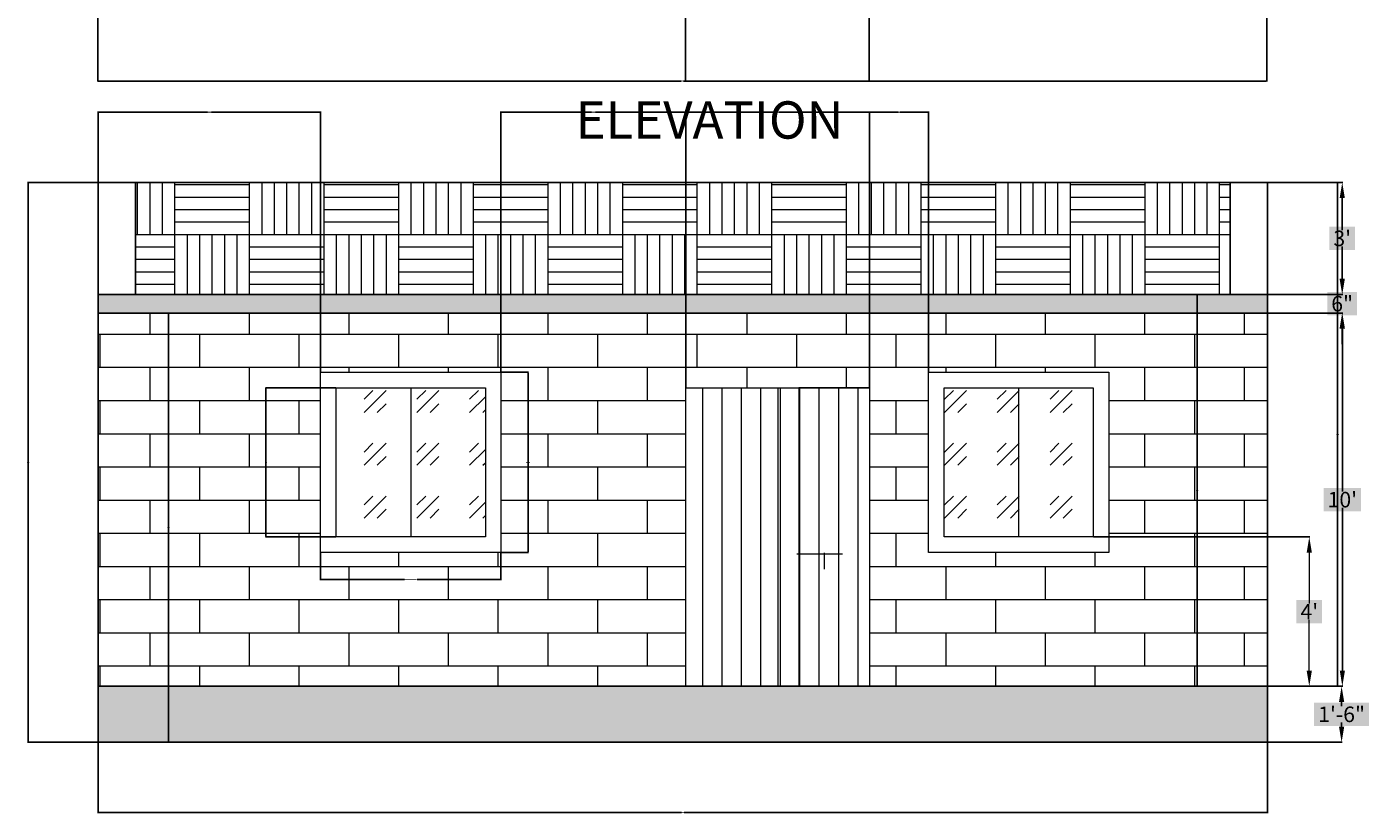
# Model space of a CAD drawing. Units: inches. Extents: x -35 to 832, y -515 to 219.
# Tile 1 of 7: x -33 to 399, y -515 to -262. Entities that reach past the tile are written whole.
import ezdxf

# ---------------------------------------------------------------- set-up
doc = ezdxf.new("R2010")
doc.units = ezdxf.units.IN
doc.header["$MEASUREMENT"] = 0
for name, color, linetype, lineweight in [('A-ANNO-DIMS', 2, 'Continuous', 18), ('A-ELEV', 3, 'Continuous', 25), ('A-ELEV-DOOR', 4, 'Continuous', 18), ('A-ELEV-GLAZ', 4, 'Continuous', 18), ('A-ELEV-PATT', 4, 'Continuous', 13), ('G-ANNO-TEXT', 7, 'Continuous', 35), ('S-ANNO-DIMS', 2, 'Continuous', 18)]:
    doc.layers.add(name, color=color, linetype=linetype, lineweight=lineweight)
doc.styles.get("Standard").update_dxf_attribs({"font": 'arial.ttf'})
doc.dimstyles.get("Standard").update_dxf_attribs({"dimtxt": 0.18, "dimasz": 0.18, "dimexe": 0.18, "dimexo": 0.0625, "dimgap": 0.09, "dimtad": 0, "dimtih": 1, "dimtoh": 1, "dimdec": 1, "dimzin": 0, "dimdsep": 46, "dimlunit": 4, "dimtxsty": 'Standard', "dimcen": 0.09, "dimclrd": 211, "dimclre": 4, "dimclrt": 3, "dimadec": 0, "dimazin": 0, "dimtfac": 0.5, "dimtdec": 1, "dimtofl": 0, "dimtmove": 0, "dimatfit": 3, "dimfxl": 1, "dimtfill": 2, "dimtfillclr": 61, "dimtolj": 1, "dimtzin": 0, "dimarcsym": 0})

# ---------------------------------------------------------------- blocks, each defined once
blk = doc.blocks.new('*D23')
at = {"layer": 'A-ANNO-DIMS', "color": 0, "lineweight": -2, "transparency": 16777216}
for p, q in [((366.05, -474.29), (390.03, -474.29)), ((389.85, -479.29), (389.85, -480.65)), ((389.85, -487.29), (389.85, -485.93)), ((366.05, -492.29), (390.03, -492.29))]:
    blk.add_line(p, q, dxfattribs=at)
at = {"layer": 'A-ANNO-DIMS', "color": 0, "transparency": 16777216}
for points in [[(389.02, -479.29), (390.68, -479.29), (389.85, -474.29)], [(389.02, -487.29), (390.68, -487.29), (389.85, -492.29)]]:
    blk.add_solid(points, dxfattribs=at)
at = {"layer": 'Defpoints', "color": 0, "transparency": 16777216}
for p in [(365.98, -474.29), (389.85, -474.29), (365.98, -492.29)]:
    blk.add_point(p, dxfattribs=at)
at = {"layer": 'A-ANNO-DIMS', "color": 0, "transparency": 16777216, "insert": (389.85, -483.29), "char_height": 5, "attachment_point": 5, "bg_fill": 1, "box_fill_scale": 1.25, "bg_fill_color": 61, "bg_fill_transparency": 0}
blk.add_mtext('\\A1;1\'-6"', dxfattribs=at)
blk = doc.blocks.new('*D24')
at = {"layer": 'A-ANNO-DIMS', "color": 0, "lineweight": -2, "transparency": 16777216}
for p, q in [((366.05, -354.29), (390.27, -354.29)), ((390.09, -359.29), (390.09, -411.65)), ((390.09, -469.29), (390.09, -416.93)), ((366.05, -474.29), (390.27, -474.29))]:
    blk.add_line(p, q, dxfattribs=at)
at = {"layer": 'A-ANNO-DIMS', "color": 0, "transparency": 16777216}
for points in [[(389.26, -359.29), (390.92, -359.29), (390.09, -354.29)], [(389.26, -469.29), (390.92, -469.29), (390.09, -474.29)]]:
    blk.add_solid(points, dxfattribs=at)
at = {"layer": 'Defpoints', "color": 0, "transparency": 16777216}
for p in [(365.98, -354.29), (390.09, -354.29), (365.98, -474.29)]:
    blk.add_point(p, dxfattribs=at)
at = {"layer": 'A-ANNO-DIMS', "color": 0, "transparency": 16777216, "insert": (390.09, -414.29), "char_height": 5, "attachment_point": 5, "bg_fill": 1, "box_fill_scale": 1.25, "bg_fill_color": 61, "bg_fill_transparency": 0}
blk.add_mtext("\\A1;10'", dxfattribs=at)
blk = doc.blocks.new('*D25')
at = {"layer": 'A-ANNO-DIMS', "color": 0, "lineweight": -2, "transparency": 16777216}
for p, q in [((390.03, -343.29), (390.03, -338.29)), ((366.05, -348.29), (390.21, -348.29)), ((366.05, -354.29), (390.21, -354.29)), ((390.03, -359.29), (390.03, -364.29))]:
    blk.add_line(p, q, dxfattribs=at)
at = {"layer": 'A-ANNO-DIMS', "color": 0, "transparency": 16777216}
for points in [[(389.2, -343.29), (390.87, -343.29), (390.03, -348.29)], [(389.2, -359.29), (390.87, -359.29), (390.03, -354.29)]]:
    blk.add_solid(points, dxfattribs=at)
at = {"layer": 'Defpoints', "color": 0, "transparency": 16777216}
for p in [(365.98, -348.29), (390.03, -348.29), (365.98, -354.29)]:
    blk.add_point(p, dxfattribs=at)
at = {"layer": 'A-ANNO-DIMS', "color": 0, "transparency": 16777216, "insert": (390.03, -351.29), "char_height": 5, "attachment_point": 5, "bg_fill": 1, "box_fill_scale": 1.25, "bg_fill_color": 61, "bg_fill_transparency": 0}
blk.add_mtext('\\A1;6"', dxfattribs=at)
blk = doc.blocks.new('*D26')
at = {"layer": 'A-ANNO-DIMS', "color": 0, "lineweight": -2, "transparency": 16777216}
for p, q in [((366.05, -312.29), (390.24, -312.29)), ((390.06, -317.29), (390.06, -327.64)), ((390.06, -343.29), (390.06, -332.93)), ((366.05, -348.29), (390.24, -348.29))]:
    blk.add_line(p, q, dxfattribs=at)
at = {"layer": 'A-ANNO-DIMS', "color": 0, "transparency": 16777216}
for points in [[(389.23, -317.29), (390.89, -317.29), (390.06, -312.29)], [(389.23, -343.29), (390.89, -343.29), (390.06, -348.29)]]:
    blk.add_solid(points, dxfattribs=at)
at = {"layer": 'Defpoints', "color": 0, "transparency": 16777216}
for p in [(365.98, -312.29), (390.06, -312.29), (365.98, -348.29)]:
    blk.add_point(p, dxfattribs=at)
at = {"layer": 'A-ANNO-DIMS', "color": 0, "transparency": 16777216, "insert": (390.06, -330.29), "char_height": 5, "attachment_point": 5, "bg_fill": 1, "box_fill_scale": 1.25, "bg_fill_color": 61, "bg_fill_transparency": 0}
blk.add_mtext("\\A1;3'", dxfattribs=at)
blk = doc.blocks.new('*D27')
at = {"layer": 'A-ANNO-DIMS', "color": 0, "lineweight": -2, "transparency": 16777216}
for p, q in [((310.05, -426.29), (379.64, -426.29)), ((311.18, -474.29), (379.64, -474.29))]:
    blk.add_line(p, q, dxfattribs=at)
at = {"layer": 'A-ANNO-DIMS', "color": 0, "lineweight": 13, "transparency": 16777216}
for p, q in [((379.46, -431.29), (379.46, -447.7)), ((379.46, -469.29), (379.46, -452.88))]:
    blk.add_line(p, q, dxfattribs=at)
at = {"layer": 'A-ANNO-DIMS', "color": 0, "transparency": 16777216}
for points in [[(378.62, -431.29), (380.29, -431.29), (379.46, -426.29)], [(378.62, -469.29), (380.29, -469.29), (379.46, -474.29)]]:
    blk.add_solid(points, dxfattribs=at)
at = {"layer": 'Defpoints', "color": 0, "transparency": 16777216}
for p in [(309.98, -426.29), (311.12, -474.29), (379.46, -474.29)]:
    blk.add_point(p, dxfattribs=at)
at = {"layer": 'A-ANNO-DIMS', "color": 0, "transparency": 16777216, "insert": (379.46, -450.29), "char_height": 5, "attachment_point": 5, "bg_fill": 1, "box_fill_scale": 1.25, "bg_fill_color": 61, "bg_fill_transparency": 0}
blk.add_mtext("\\A1;4'", dxfattribs=at)
blk = doc.blocks.new('WIN-48-ELEV')
blk.add_line((29, 53), (29, 5))
for points in [[(0, 58), (58, 58), (58, 0), (0, 0)], [(5, 53), (53, 53), (53, 5), (5, 5)]]:
    blk.add_lwpolyline(points, close=True)
blk = doc.blocks.new('*D69')
at = {"layer": 'Defpoints', "color": 0, "transparency": 16777216}
for p in [(61.48, -431.29), (119.48, -431.29), (119.48, -439.99)]:
    blk.add_point(p, dxfattribs=at)
at = {"layer": 'S-ANNO-DIMS', "color": 4, "lineweight": -2, "transparency": 16777216}
for p, q in [((61.48, -431.35), (61.48, -440.17)), ((119.48, -431.35), (119.48, -440.17))]:
    blk.add_line(p, q, dxfattribs=at)
at = {"layer": 'S-ANNO-DIMS', "color": 211, "lineweight": -2, "transparency": 16777216}
for p, q in [((61.66, -439.99), (88.42, -439.99)), ((119.3, -439.99), (92.54, -439.99))]:
    blk.add_line(p, q, dxfattribs=at)
at = {"layer": 'S-ANNO-DIMS', "color": 211, "transparency": 16777216}
for points in [[(61.66, -439.96), (61.66, -440.02), (61.48, -439.99)], [(119.3, -439.96), (119.3, -440.02), (119.48, -439.99)]]:
    blk.add_solid(points, dxfattribs=at)
at = {"layer": 'S-ANNO-DIMS', "color": 3, "transparency": 16777216, "insert": (90.48, -439.99), "char_height": 0.18, "attachment_point": 5, "bg_fill": 1, "box_fill_scale": 1.25, "bg_fill_color": 61, "bg_fill_transparency": 0}
blk.add_mtext('\\A1;WINDOW SURROUND 4\'-10" TYP.', dxfattribs=at)
blk = doc.blocks.new('*D70')
at = {"layer": 'Defpoints', "color": 0, "transparency": 16777216}
for p in [(119.48, -373.29), (128.18, -373.29), (119.48, -431.29)]:
    blk.add_point(p, dxfattribs=at)
at = {"layer": 'S-ANNO-DIMS', "color": 4, "lineweight": -2, "transparency": 16777216}
for p, q in [((119.55, -373.29), (128.36, -373.29)), ((119.55, -431.29), (128.36, -431.29))]:
    blk.add_line(p, q, dxfattribs=at)
at = {"layer": 'S-ANNO-DIMS', "color": 211, "lineweight": -2, "transparency": 16777216}
for p, q in [((128.18, -373.47), (128.18, -402.11)), ((128.18, -431.11), (128.18, -402.47))]:
    blk.add_line(p, q, dxfattribs=at)
at = {"layer": 'S-ANNO-DIMS', "color": 211, "transparency": 16777216}
for points in [[(128.15, -373.47), (128.21, -373.47), (128.18, -373.29)], [(128.15, -431.11), (128.21, -431.11), (128.18, -431.29)]]:
    blk.add_solid(points, dxfattribs=at)
at = {"layer": 'S-ANNO-DIMS', "color": 3, "transparency": 16777216, "insert": (128.18, -402.29), "char_height": 0.18, "attachment_point": 5, "bg_fill": 1, "box_fill_scale": 1.25, "bg_fill_color": 61, "bg_fill_transparency": 0}
blk.add_mtext('\\A1;4\'-10" TYP.', dxfattribs=at)
blk = doc.blocks.new('*D109')
at = {"layer": 'Defpoints', "color": 0, "transparency": 16777216}
for p in [(365.8, -100.95), (-10.2, -143.45), (365.8, -279.7)]:
    blk.add_point(p, dxfattribs=at)
at = {"layer": 'S-ANNO-DIMS', "color": 4, "lineweight": -2, "transparency": 16777216}
for p, q in [((365.8, -101.01), (365.8, -279.88)), ((-10.2, -143.51), (-10.2, -279.88))]:
    blk.add_line(p, q, dxfattribs=at)
at = {"layer": 'S-ANNO-DIMS', "color": 211, "lineweight": -2, "transparency": 16777216}
for p, q in [((-10.02, -279.7), (177.4, -279.7)), ((365.62, -279.7), (178.2, -279.7))]:
    blk.add_line(p, q, dxfattribs=at)
at = {"layer": 'S-ANNO-DIMS', "color": 211, "transparency": 16777216}
for points in [[(-10.02, -279.67), (-10.02, -279.73), (-10.2, -279.7)], [(365.62, -279.67), (365.62, -279.73), (365.8, -279.7)]]:
    blk.add_solid(points, dxfattribs=at)
at = {"layer": 'S-ANNO-DIMS', "color": 3, "transparency": 16777216, "insert": (177.8, -279.7), "char_height": 0.18, "attachment_point": 5, "bg_fill": 1, "box_fill_scale": 1.25, "bg_fill_color": 61, "bg_fill_transparency": 0}
blk.add_mtext('\\A1;31\'-4"', dxfattribs=at)
blk = doc.blocks.new('*D111')
at = {"layer": 'Defpoints', "color": 0, "transparency": 16777216}
for p in [(178.8, -149.95), (237.86, -149.95), (237.86, -279.7)]:
    blk.add_point(p, dxfattribs=at)
at = {"layer": 'S-ANNO-DIMS', "color": 4, "lineweight": -2, "transparency": 16777216}
for p, q in [((178.8, -150.01), (178.8, -279.88)), ((237.86, -150.01), (237.86, -279.88))]:
    blk.add_line(p, q, dxfattribs=at)
at = {"layer": 'S-ANNO-DIMS', "color": 211, "lineweight": -2, "transparency": 16777216}
for p, q in [((178.98, -279.7), (207.93, -279.7)), ((237.68, -279.7), (208.73, -279.7))]:
    blk.add_line(p, q, dxfattribs=at)
at = {"layer": 'S-ANNO-DIMS', "color": 211, "transparency": 16777216}
for points in [[(178.98, -279.67), (178.98, -279.73), (178.8, -279.7)], [(237.68, -279.67), (237.68, -279.73), (237.86, -279.7)]]:
    blk.add_solid(points, dxfattribs=at)
at = {"layer": 'S-ANNO-DIMS', "color": 3, "transparency": 16777216, "insert": (208.33, -279.7), "char_height": 0.18, "attachment_point": 5, "bg_fill": 1, "box_fill_scale": 1.25, "bg_fill_color": 61, "bg_fill_transparency": 0}
blk.add_mtext('\\A1;4\'-11"', dxfattribs=at)
blk = doc.blocks.new('*D125')
at = {"layer": 'Defpoints', "color": 0, "transparency": 16777216}
for p in [(61.48, -289.69), (-10.02, -312.29), (61.48, -373.29)]:
    blk.add_point(p, dxfattribs=at)
at = {"layer": 'S-ANNO-DIMS', "color": 4, "lineweight": -2, "transparency": 16777216}
for p, q in [((-10.02, -312.23), (-10.02, -289.51)), ((61.48, -373.23), (61.48, -289.51))]:
    blk.add_line(p, q, dxfattribs=at)
at = {"layer": 'S-ANNO-DIMS', "color": 211, "lineweight": -2, "transparency": 16777216}
for p, q in [((-9.84, -289.69), (25.12, -289.69)), ((61.3, -289.69), (26.34, -289.69))]:
    blk.add_line(p, q, dxfattribs=at)
at = {"layer": 'S-ANNO-DIMS', "color": 211, "transparency": 16777216}
for points in [[(-9.84, -289.66), (-9.84, -289.72), (-10.02, -289.69)], [(61.3, -289.66), (61.3, -289.72), (61.48, -289.69)]]:
    blk.add_solid(points, dxfattribs=at)
at = {"layer": 'S-ANNO-DIMS', "color": 3, "transparency": 16777216, "insert": (25.73, -289.69), "char_height": 0.18, "attachment_point": 5, "bg_fill": 1, "box_fill_scale": 1.25, "bg_fill_color": 61, "bg_fill_transparency": 0}
blk.add_mtext('\\A1;5\'-11 1/2"', dxfattribs=at)
blk = doc.blocks.new('*D126')
at = {"layer": 'Defpoints', "color": 0, "transparency": 16777216}
for p in [(178.98, -289.69), (119.48, -373.29), (178.98, -378.29)]:
    blk.add_point(p, dxfattribs=at)
at = {"layer": 'S-ANNO-DIMS', "color": 4, "lineweight": -2, "transparency": 16777216}
for p, q in [((119.48, -373.23), (119.48, -289.51)), ((178.98, -378.23), (178.98, -289.51))]:
    blk.add_line(p, q, dxfattribs=at)
at = {"layer": 'S-ANNO-DIMS', "color": 211, "lineweight": -2, "transparency": 16777216}
for p, q in [((119.66, -289.69), (148.62, -289.69)), ((178.8, -289.69), (149.85, -289.69))]:
    blk.add_line(p, q, dxfattribs=at)
at = {"layer": 'S-ANNO-DIMS', "color": 211, "transparency": 16777216}
for points in [[(119.66, -289.66), (119.66, -289.72), (119.48, -289.69)], [(178.8, -289.66), (178.8, -289.72), (178.98, -289.69)]]:
    blk.add_solid(points, dxfattribs=at)
at = {"layer": 'S-ANNO-DIMS', "color": 3, "transparency": 16777216, "insert": (149.23, -289.69), "char_height": 0.18, "attachment_point": 5, "bg_fill": 1, "box_fill_scale": 1.25, "bg_fill_color": 61, "bg_fill_transparency": 0}
blk.add_mtext('\\A1;4\'-11 1/2"', dxfattribs=at)
blk = doc.blocks.new('*D127')
at = {"layer": 'Defpoints', "color": 0, "transparency": 16777216}
for p in [(238.04, -289.69), (178.98, -378.29), (238.04, -378.29)]:
    blk.add_point(p, dxfattribs=at)
at = {"layer": 'S-ANNO-DIMS', "color": 4, "lineweight": -2, "transparency": 16777216}
for p, q in [((178.98, -378.23), (178.98, -289.51)), ((238.04, -378.23), (238.04, -289.51))]:
    blk.add_line(p, q, dxfattribs=at)
at = {"layer": 'S-ANNO-DIMS', "color": 211, "lineweight": -2, "transparency": 16777216}
for p, q in [((179.16, -289.69), (208.11, -289.69)), ((237.86, -289.69), (208.91, -289.69))]:
    blk.add_line(p, q, dxfattribs=at)
at = {"layer": 'S-ANNO-DIMS', "color": 211, "transparency": 16777216}
for points in [[(179.16, -289.66), (179.16, -289.72), (178.98, -289.69)], [(237.86, -289.66), (237.86, -289.72), (238.04, -289.69)]]:
    blk.add_solid(points, dxfattribs=at)
at = {"layer": 'S-ANNO-DIMS', "color": 3, "transparency": 16777216, "insert": (208.51, -289.69), "char_height": 0.18, "attachment_point": 5, "bg_fill": 1, "box_fill_scale": 1.25, "bg_fill_color": 61, "bg_fill_transparency": 0}
blk.add_mtext('\\A1;4\'-11"', dxfattribs=at)
blk = doc.blocks.new('*D128')
at = {"layer": 'Defpoints', "color": 0, "transparency": 16777216}
for p in [(256.98, -289.69), (256.98, -373.29), (238.04, -378.29)]:
    blk.add_point(p, dxfattribs=at)
at = {"layer": 'S-ANNO-DIMS', "color": 4, "lineweight": -2, "transparency": 16777216}
for p, q in [((238.04, -378.23), (238.04, -289.51)), ((256.98, -373.23), (256.98, -289.51))]:
    blk.add_line(p, q, dxfattribs=at)
at = {"layer": 'S-ANNO-DIMS', "color": 211, "lineweight": -2, "transparency": 16777216}
for p, q in [((238.22, -289.69), (247.19, -289.69)), ((256.8, -289.69), (247.83, -289.69))]:
    blk.add_line(p, q, dxfattribs=at)
at = {"layer": 'S-ANNO-DIMS', "color": 211, "transparency": 16777216}
for points in [[(238.22, -289.66), (238.22, -289.72), (238.04, -289.69)], [(256.8, -289.66), (256.8, -289.72), (256.98, -289.69)]]:
    blk.add_solid(points, dxfattribs=at)
at = {"layer": 'S-ANNO-DIMS', "color": 3, "transparency": 16777216, "insert": (247.51, -289.69), "char_height": 0.18, "attachment_point": 5, "bg_fill": 1, "box_fill_scale": 1.25, "bg_fill_color": 61, "bg_fill_transparency": 0}
blk.add_mtext('\\A1;1\'-7"', dxfattribs=at)
blk = doc.blocks.new('*D129')
at = {"layer": 'Defpoints', "color": 0, "transparency": 16777216}
for p in [(215.44, -378.29), (238.04, -378.29), (238.04, -474.29)]:
    blk.add_point(p, dxfattribs=at)
at = {"layer": 'S-ANNO-DIMS', "color": 4, "lineweight": -2, "transparency": 16777216}
for p, q in [((237.98, -378.29), (215.26, -378.29)), ((237.98, -474.29), (215.26, -474.29))]:
    blk.add_line(p, q, dxfattribs=at)
at = {"layer": 'S-ANNO-DIMS', "color": 211, "lineweight": -2, "transparency": 16777216}
for p, q in [((215.44, -378.47), (215.44, -426.11)), ((215.44, -474.11), (215.44, -426.47))]:
    blk.add_line(p, q, dxfattribs=at)
at = {"layer": 'S-ANNO-DIMS', "color": 211, "transparency": 16777216}
for points in [[(215.41, -378.47), (215.47, -378.47), (215.44, -378.29)], [(215.41, -474.11), (215.47, -474.11), (215.44, -474.29)]]:
    blk.add_solid(points, dxfattribs=at)
at = {"layer": 'S-ANNO-DIMS', "color": 3, "transparency": 16777216, "insert": (215.44, -426.29), "char_height": 0.18, "attachment_point": 5, "bg_fill": 1, "box_fill_scale": 1.25, "bg_fill_color": 61, "bg_fill_transparency": 0}
blk.add_mtext('\\A1;8\'-0"', dxfattribs=at)
blk = doc.blocks.new('*D130')
at = {"layer": 'Defpoints', "color": 0, "transparency": 16777216}
for p in [(-10.02, -492.29), (365.98, -492.29), (365.98, -514.89)]:
    blk.add_point(p, dxfattribs=at)
at = {"layer": 'S-ANNO-DIMS', "color": 4, "lineweight": -2, "transparency": 16777216}
for p, q in [((-10.02, -492.35), (-10.02, -515.07)), ((365.98, -492.35), (365.98, -515.07))]:
    blk.add_line(p, q, dxfattribs=at)
at = {"layer": 'S-ANNO-DIMS', "color": 211, "lineweight": -2, "transparency": 16777216}
for p, q in [((-9.84, -514.89), (177.58, -514.89)), ((365.8, -514.89), (178.38, -514.89))]:
    blk.add_line(p, q, dxfattribs=at)
at = {"layer": 'S-ANNO-DIMS', "color": 211, "transparency": 16777216}
for points in [[(-9.84, -514.86), (-9.84, -514.92), (-10.02, -514.89)], [(365.8, -514.86), (365.8, -514.92), (365.98, -514.89)]]:
    blk.add_solid(points, dxfattribs=at)
at = {"layer": 'S-ANNO-DIMS', "color": 3, "transparency": 16777216, "insert": (177.98, -514.89), "char_height": 0.18, "attachment_point": 5, "bg_fill": 1, "box_fill_scale": 1.25, "bg_fill_color": 61, "bg_fill_transparency": 0}
blk.add_mtext('\\A1;31\'-4"', dxfattribs=at)
blk = doc.blocks.new('*D131')
at = {"layer": 'Defpoints', "color": 0, "transparency": 16777216}
for p in [(-32.62, -312.29), (-10.02, -312.29), (-10.02, -492.29)]:
    blk.add_point(p, dxfattribs=at)
at = {"layer": 'S-ANNO-DIMS', "color": 4, "lineweight": -2, "transparency": 16777216}
for p, q in [((-10.08, -312.29), (-32.8, -312.29)), ((-10.08, -492.29), (-32.8, -492.29))]:
    blk.add_line(p, q, dxfattribs=at)
at = {"layer": 'S-ANNO-DIMS', "color": 211, "lineweight": -2, "transparency": 16777216}
for p, q in [((-32.62, -312.47), (-32.62, -402.11)), ((-32.62, -492.11), (-32.62, -402.47))]:
    blk.add_line(p, q, dxfattribs=at)
at = {"layer": 'S-ANNO-DIMS', "color": 211, "transparency": 16777216}
for points in [[(-32.65, -312.47), (-32.59, -312.47), (-32.62, -312.29)], [(-32.65, -492.11), (-32.59, -492.11), (-32.62, -492.29)]]:
    blk.add_solid(points, dxfattribs=at)
at = {"layer": 'S-ANNO-DIMS', "color": 3, "transparency": 16777216, "insert": (-32.62, -402.29), "char_height": 0.18, "attachment_point": 5, "bg_fill": 1, "box_fill_scale": 1.25, "bg_fill_color": 61, "bg_fill_transparency": 0}
blk.add_mtext('\\A1;15\'-0"', dxfattribs=at)
blk = doc.blocks.new('*D132')
at = {"layer": 'Defpoints', "color": 0, "transparency": 16777216}
for p in [(365.98, -312.29), (365.98, -474.29), (388.58, -474.29)]:
    blk.add_point(p, dxfattribs=at)
at = {"layer": 'S-ANNO-DIMS', "color": 4, "lineweight": -2, "transparency": 16777216}
for p, q in [((366.05, -312.29), (388.76, -312.29)), ((366.05, -474.29), (388.76, -474.29))]:
    blk.add_line(p, q, dxfattribs=at)
at = {"layer": 'S-ANNO-DIMS', "color": 211, "lineweight": -2, "transparency": 16777216}
for p, q in [((388.58, -312.47), (388.58, -393.11)), ((388.58, -474.11), (388.58, -393.47))]:
    blk.add_line(p, q, dxfattribs=at)
at = {"layer": 'S-ANNO-DIMS', "color": 211, "transparency": 16777216}
for points in [[(388.55, -312.47), (388.61, -312.47), (388.58, -312.29)], [(388.55, -474.11), (388.61, -474.11), (388.58, -474.29)]]:
    blk.add_solid(points, dxfattribs=at)
at = {"layer": 'S-ANNO-DIMS', "color": 3, "transparency": 16777216, "insert": (388.58, -393.29), "char_height": 0.18, "attachment_point": 5, "bg_fill": 1, "box_fill_scale": 1.25, "bg_fill_color": 61, "bg_fill_transparency": 0}
blk.add_mtext('\\A1;13\'-6"', dxfattribs=at)
blk = doc.blocks.new('*D133')
at = {"layer": 'Defpoints', "color": 0, "transparency": 16777216}
for p in [(-10.02, -354.29), (-10.02, -492.29), (12.58, -492.29)]:
    blk.add_point(p, dxfattribs=at)
at = {"layer": 'S-ANNO-DIMS', "color": 4, "lineweight": -2, "transparency": 16777216}
for p, q in [((-9.95, -354.29), (12.76, -354.29)), ((-9.95, -492.29), (12.76, -492.29))]:
    blk.add_line(p, q, dxfattribs=at)
at = {"layer": 'S-ANNO-DIMS', "color": 211, "lineweight": -2, "transparency": 16777216}
for p, q in [((12.58, -354.47), (12.58, -423.11)), ((12.58, -492.11), (12.58, -423.47))]:
    blk.add_line(p, q, dxfattribs=at)
at = {"layer": 'S-ANNO-DIMS', "color": 211, "transparency": 16777216}
for points in [[(12.55, -354.47), (12.61, -354.47), (12.58, -354.29)], [(12.55, -492.11), (12.61, -492.11), (12.58, -492.29)]]:
    blk.add_solid(points, dxfattribs=at)
at = {"layer": 'S-ANNO-DIMS', "color": 3, "transparency": 16777216, "insert": (12.58, -423.29), "char_height": 0.18, "attachment_point": 5, "bg_fill": 1, "box_fill_scale": 1.25, "bg_fill_color": 61, "bg_fill_transparency": 0}
blk.add_mtext('\\A1;11\'-6"', dxfattribs=at)
blk = doc.blocks.new('*D134')
at = {"layer": 'Defpoints', "color": 0, "transparency": 16777216}
for p in [(343.38, -348.29), (365.98, -348.29), (365.98, -474.29)]:
    blk.add_point(p, dxfattribs=at)
at = {"layer": 'S-ANNO-DIMS', "color": 4, "lineweight": -2, "transparency": 16777216}
for p, q in [((365.92, -348.29), (343.2, -348.29)), ((365.92, -474.29), (343.2, -474.29))]:
    blk.add_line(p, q, dxfattribs=at)
at = {"layer": 'S-ANNO-DIMS', "color": 211, "lineweight": -2, "transparency": 16777216}
for p, q in [((343.38, -348.47), (343.38, -411.11)), ((343.38, -474.11), (343.38, -411.47))]:
    blk.add_line(p, q, dxfattribs=at)
at = {"layer": 'S-ANNO-DIMS', "color": 211, "transparency": 16777216}
for points in [[(343.35, -348.47), (343.41, -348.47), (343.38, -348.29)], [(343.35, -474.11), (343.41, -474.11), (343.38, -474.29)]]:
    blk.add_solid(points, dxfattribs=at)
at = {"layer": 'S-ANNO-DIMS', "color": 3, "transparency": 16777216, "insert": (343.38, -411.29), "char_height": 0.18, "attachment_point": 5, "bg_fill": 1, "box_fill_scale": 1.25, "bg_fill_color": 61, "bg_fill_transparency": 0}
blk.add_mtext('\\A1;10\'-6"', dxfattribs=at)
blk = doc.blocks.new('*D135')
at = {"layer": 'Defpoints', "color": 0, "transparency": 16777216}
for p in [(43.88, -378.29), (66.48, -378.29), (66.48, -426.29)]:
    blk.add_point(p, dxfattribs=at)
at = {"layer": 'S-ANNO-DIMS', "color": 4, "lineweight": -2, "transparency": 16777216}
for p, q in [((66.42, -378.29), (43.7, -378.29)), ((66.42, -426.29), (43.7, -426.29))]:
    blk.add_line(p, q, dxfattribs=at)
at = {"layer": 'S-ANNO-DIMS', "color": 211, "lineweight": -2, "transparency": 16777216}
for p, q in [((43.88, -378.47), (43.88, -402.11)), ((43.88, -426.11), (43.88, -402.47))]:
    blk.add_line(p, q, dxfattribs=at)
at = {"layer": 'S-ANNO-DIMS', "color": 211, "transparency": 16777216}
for points in [[(43.85, -378.47), (43.91, -378.47), (43.88, -378.29)], [(43.85, -426.11), (43.91, -426.11), (43.88, -426.29)]]:
    blk.add_solid(points, dxfattribs=at)
at = {"layer": 'S-ANNO-DIMS', "color": 3, "transparency": 16777216, "insert": (43.88, -402.29), "char_height": 0.18, "attachment_point": 5, "bg_fill": 1, "box_fill_scale": 1.25, "bg_fill_color": 61, "bg_fill_transparency": 0}
blk.add_mtext('\\A1;4\'-0"', dxfattribs=at)

msp = doc.modelspace()

# ---------------------------------------------------------------- hatches: boundary and pattern name
at = {"layer": 'A-ELEV-PATT'}
h = msp.add_hatch(dxfattribs=at)
h.set_pattern_fill('AR-PARQ1', color=256, scale=2)
h.set_pattern_definition([(90, (-9.392, 54.963), (-24, 24), [24, -24]), (90, (-5.392, 54.963), (-24, 24), [24, -24]), (90, (-1.392, 54.963), (-24, 24), [24, -24]), (90, (2.608, 54.963), (-24, 24), [24, -24]), (90, (6.608, 54.963), (-24, 24), [24, -24]), (90, (10.608, 54.963), (-24, 24), [24, -24]), (90, (14.608, 54.963), (-24, 24), [24, -24]), (0, (-9.392, 78.963), (24, -24), [24, -24]), (0, (-9.392, 82.963), (24, -24), [24, -24]), (0, (-9.392, 86.963), (24, -24), [24, -24]), (0, (-9.392, 90.963), (24, -24), [24, -24]), (0, (-9.392, 94.963), (24, -24), [24, -24]), (0, (-9.392, 98.963), (24, -24), [24, -24]), (0, (-9.392, 102.963), (24, -24), [24, -24])])
h.paths.add_polyline_path([(1.98, -312.29), (1.98, -348.29), (353.98, -348.29), (353.98, -312.29)])
h = msp.add_hatch(color=256, dxfattribs=at)
h.dxf.hatch_style = 1
h.paths.add_polyline_path([(365.98, -354.29), (365.98, -348.29), (-10.02, -348.29), (-10.02, -354.29)])
h = msp.add_hatch(dxfattribs=at)
h.set_pattern_fill('AR-BRSTD', color=256, scale=4)
h.set_pattern_definition([(0, (-9.392, 54.963), (0, 10.668), []), (90, (-9.392, 54.963), (-16, 10.668), [10.668, -10.668])])
h.paths.add_polyline_path([(178.98, -378.29), (238.04, -378.29), (238.04, -474.29), (365.98, -474.29), (365.98, -354.29), (-10.02, -354.29), (-10.02, -474.29), (178.98, -474.29)])
h.paths.add_polyline_path([(61.48, -373.29), (119.48, -373.29), (119.48, -431.29), (61.48, -431.29)], flags=16)
h.paths.add_polyline_path([(66.48, -378.29), (114.48, -378.29), (114.48, -426.29), (66.48, -426.29)], flags=0)
h.paths.add_polyline_path([(256.98, -373.29), (314.98, -373.29), (314.98, -431.29), (256.98, -431.29)], flags=16)
h.paths.add_polyline_path([(261.98, -378.29), (309.98, -378.29), (309.98, -426.29), (261.98, -426.29)], flags=0)
h = msp.add_hatch(dxfattribs=at)
h.set_pattern_fill('GOST_GLASS', color=256, scale=2)
h.set_pattern_definition([(45, (-9.392, 54.963), (16.97056, -2e-15), [10, -14]), (45, (-5.149, 54.963), (16.97056, -2e-15), [4, -20]), (45, (-9.392, 59.206), (16.97056, -2e-15), [4, -20])])
h.paths.add_polyline_path([(90.48, -378.29), (66.48, -378.29), (66.48, -426.29), (90.48, -426.29)])
h.paths.add_polyline_path([(114.48, -378.29), (90.48, -378.29), (90.48, -426.29), (114.48, -426.29)])
h.paths.add_polyline_path([(285.98, -378.29), (261.98, -378.29), (261.98, -426.29), (285.98, -426.29)])
h.paths.add_polyline_path([(309.98, -378.29), (285.98, -378.29), (285.98, -426.29), (309.98, -426.29)])
h = msp.add_hatch(dxfattribs=at)
h.set_pattern_fill('ANSI31', color=256, scale=50, angle=45)
h.set_pattern_definition([(90, (-9.392, 54.963), (-6.25, 1e-15), [])])
h.paths.add_polyline_path([(208.51, -378.29), (178.98, -378.29), (178.98, -474.29), (208.51, -474.29)])
h.paths.add_polyline_path([(238.04, -378.29), (208.51, -378.29), (208.51, -474.29), (238.04, -474.29)])
h = msp.add_hatch(dxfattribs=at)
h.set_pattern_fill('AR-CONC', color=256, scale=2)
h.set_pattern_definition([(50, (-9.392, 54.963), (14.3452, -1.25504), [1.5, -16.5]), (355, (-9.392, 54.963), (-2.77503, 15.04384), [1.2, -13.2]), (100.4514, (-8.196, 54.859), (11.57018, 13.7888), [1.2748, -14.02284]), (46.1842, (-9.392, 58.963), (21.34483, -3.3104), [2.25, -24.75]), (96.6356, (-7.613, 58.687), (18.69324, 19.4824), [1.9122, -21.0343]), (351.184, (-9.392, 58.963), (18.69324, 19.4824), [1.8, -19.8]), (21, (-7.392, 57.963), (11.93814, -8.05238), [1.5, -16.5]), (326, (-7.392, 57.963), (4.8663, 14.503), [1.2, -13.2]), (71.4514, (-6.397, 57.292), (16.80445, 6.45062), [1.2748, -14.02284]), (37.5, (-9.392, 54.963), (0.243197, 6.657877), [0, -13.04, 0, -13.4, 0, -13.25]), (7.5, (-9.392, 54.963), (5.26139, 7.888234), [0, -7.64, 0, -12.74, 0, -5.05]), (327.5, (-13.852, 54.963), (10.67645, -0.451097), [0, -5, 0, -15.6, 0, -20.7]), (317.5, (-15.852, 54.963), (11.66372, 2.0021), [0, -6.5, 0, -10.36, 0, -14.7])])
h.paths.add_polyline_path([(-10.02, -474.29), (-10.02, -492.29), (365.98, -492.29), (365.98, -474.29)])

# ---------------------------------------------------------------- linework, layer by layer
at = {"layer": 'A-ELEV'}
for p, q in [((-10.02, -312.29), (365.98, -312.29)), ((1.98, -312.29), (1.98, -348.29)), ((353.98, -312.29), (353.98, -348.29)), ((-10.02, -348.29), (365.98, -348.29)), ((-10.02, -354.29), (365.98, -354.29)), ((-10.02, -474.29), (365.98, -474.29)), ((-10.02, -492.29), (365.98, -492.29))]:
    msp.add_line(p, q, dxfattribs=at)
for points in [[(-10.02, -312.29), (365.98, -312.29), (365.98, -348.29), (-10.02, -348.29)], [(-10.02, -348.29), (365.98, -348.29), (365.98, -354.29), (-10.02, -354.29)], [(-10.02, -354.29), (365.98, -354.29), (365.98, -474.29), (-10.02, -474.29)], [(-10.02, -474.29), (365.98, -474.29), (365.98, -492.29), (-10.02, -492.29)]]:
    msp.add_lwpolyline(points, close=True, dxfattribs=at)
at = {"layer": 'A-ELEV-DOOR'}
for p, q in [((208.51, -378.29), (208.51, -474.29)), ((223.38, -431.38), (223.38, -436.66)), ((214.69, -431.72), (229.34, -431.72))]:
    msp.add_line(p, q, dxfattribs=at)
msp.add_lwpolyline([(178.98, -378.29), (238.04, -378.29), (238.04, -474.29), (178.98, -474.29)], close=True, dxfattribs=at)

# ---------------------------------------------------------------- block references
at = {"layer": 'A-ELEV-GLAZ'}
for p in [(61.48, -431.29), (256.98, -431.29)]:
    msp.add_blockref('WIN-48-ELEV', p, dxfattribs=at)

# ---------------------------------------------------------------- texts
at = {"layer": 'G-ANNO-TEXT', "insert": (143.51, -286.23), "char_height": 12, "attachment_point": 1}
msp.add_mtext_dynamic_manual_height_columns('ELEVATION', width=219.0757, gutter_width=1, heights=[0], dxfattribs=at)

# ---------------------------------------------------------------- dimensions: what is measured, and where the dimension line sits
at = {"layer": 'A-ANNO-DIMS'}
for base, p1, p2, override, picture, middle in [((390.06, -312.29), (365.98, -348.29), (365.98, -312.29), {"dimtxt": 5, "dimasz": 5, "dimclrd": 0, "dimclre": 0, "dimclrt": 0}, '*D26', (390.06, -330.29)), ((390.03, -348.29), (365.98, -354.29), (365.98, -348.29), {"dimtxt": 5, "dimasz": 5, "dimclrd": 0, "dimclre": 0, "dimclrt": 0}, '*D25', (390.03, -351.29)), ((390.09, -354.29), (365.98, -474.29), (365.98, -354.29), {"dimtxt": 5, "dimasz": 5, "dimclrd": 0, "dimclre": 0, "dimclrt": 0}, '*D24', (390.09, -414.29)), ((379.46, -474.29), (309.98, -426.29), (311.12, -474.29), {"dimtxt": 5, "dimasz": 5, "dimclrd": 0, "dimclre": 0, "dimclrt": 0, "dimlwd": 13}, '*D27', (379.46, -450.29)), ((389.85, -474.29), (365.98, -492.29), (365.98, -474.29), {"dimtxt": 5, "dimasz": 5, "dimclrd": 0, "dimclre": 0, "dimclrt": 0}, '*D23', (389.85, -483.29))]:
    dim = msp.add_linear_dim(base=base, p1=p1, p2=p2, angle=90, dimstyle='Standard', override=override, dxfattribs=at)
    dim.commit()
    dim.dimension.update_dxf_attribs({"geometry": picture, "text_midpoint": middle})
at = {"layer": 'S-ANNO-DIMS'}
for base, p1, p2, picture, middle in [((365.8, -279.7), (-10.2, -143.45), (365.8, -100.95), '*D109', (177.8, -279.7)), ((237.86, -279.7), (178.8, -149.95), (237.86, -149.95), '*D111', (208.33, -279.7)), ((61.48, -289.69), (-10.02, -312.29), (61.48, -373.29), '*D125', (25.73, -289.69)), ((178.98, -289.69), (119.48, -373.29), (178.98, -378.29), '*D126', (149.23, -289.69)), ((238.04, -289.69), (178.98, -378.29), (238.04, -378.29), '*D127', (208.51, -289.69)), ((256.98, -289.69), (238.04, -378.29), (256.98, -373.29), '*D128', (247.51, -289.69)), ((365.98, -514.89), (-10.02, -492.29), (365.98, -492.29), '*D130', (177.98, -514.89))]:
    dim = msp.add_linear_dim(base=base, p1=p1, p2=p2, dimstyle='Standard', override={"dimdec": 1, "dimlfac": 1, "dimrnd": 0, "dimzin": 1, "dimdsep": 46, "dimlunit": 4, "dimfrac": 2}, dxfattribs=at)
    dim.commit()
    dim.dimension.update_dxf_attribs({"geometry": picture, "text_midpoint": middle})
for base, p1, p2, angle, picture, middle in [((-32.62, -312.29), (-10.02, -492.29), (-10.02, -312.29), 90, '*D131', (-32.62, -402.29)), ((388.58, -474.29), (365.98, -312.29), (365.98, -474.29), 270, '*D132', (388.58, -393.29)), ((343.38, -348.29), (365.98, -474.29), (365.98, -348.29), 90, '*D134', (343.38, -411.29)), ((12.58, -492.29), (-10.02, -354.29), (-10.02, -492.29), 270, '*D133', (12.58, -423.29)), ((43.88, -378.29), (66.48, -426.29), (66.48, -378.29), 90, '*D135', (43.88, -402.29)), ((215.44, -378.29), (238.04, -474.29), (238.04, -378.29), 90, '*D129', (215.44, -426.29))]:
    dim = msp.add_linear_dim(base=base, p1=p1, p2=p2, angle=angle, dimstyle='Standard', override={"dimdec": 1, "dimlfac": 1, "dimrnd": 0, "dimzin": 1, "dimdsep": 46, "dimlunit": 4, "dimfrac": 2}, dxfattribs=at)
    dim.commit()
    dim.dimension.update_dxf_attribs({"geometry": picture, "text_midpoint": middle})
dim = msp.add_linear_dim(base=(128.18, -373.29), p1=(119.48, -431.29), p2=(119.48, -373.29), angle=90, text='<> TYP.', dimstyle='Standard', override={"dimdec": 1, "dimlfac": 1, "dimrnd": 0, "dimzin": 1, "dimdsep": 46, "dimlunit": 4, "dimfrac": 2}, dxfattribs=at)
dim.commit()
dim.dimension.update_dxf_attribs({"geometry": '*D70', "text_midpoint": (128.18, -402.29)})
dim = msp.add_linear_dim(base=(119.48, -439.99), p1=(61.48, -431.29), p2=(119.48, -431.29), text='WINDOW SURROUND <> TYP.', dimstyle='Standard', override={"dimdec": 1, "dimlfac": 1, "dimrnd": 0, "dimzin": 1, "dimdsep": 46, "dimlunit": 4, "dimfrac": 2}, dxfattribs=at)
dim.commit()
dim.dimension.update_dxf_attribs({"geometry": '*D69', "text_midpoint": (90.48, -439.99)})

doc.saveas('drawing.dxf')
